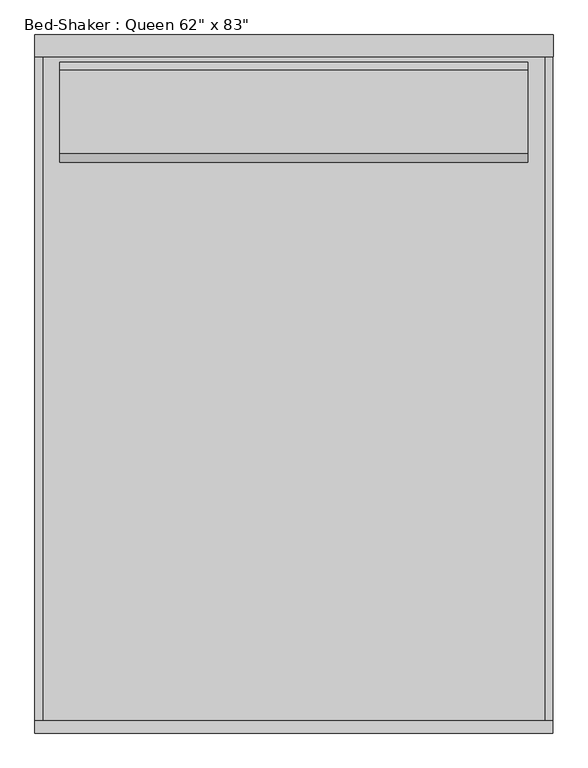
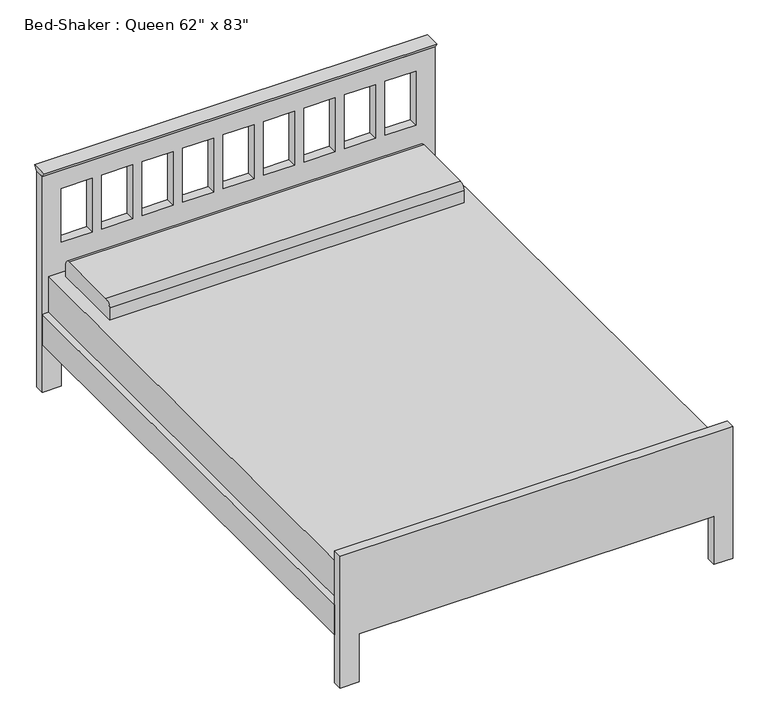
"""IFC4 building model written with IfcOpenShell, lengths in millimetres: furniture geometry."""

from ifc_helpers import new_model, si_unit, point, frame, frame_2d, origin, place, context, project, spatial, polyline, circle_curve, trimmed, segment, composite_curve, outline, extrude, source, transform, mapped, element, save


def furniture_35c09872(model_context):
    return source(origin(), model_context, "Body", "SweptSolid", [
        extrude(outline(polyline([(-38.1, 914.4), (-51.9545455, 933.45), (13.8545455, 933.45), (0.0, 914.4), (-38.1, 914.4)])), frame((-806.2365546, 0.0, 0.0), z_axis=(1.0, 0.0, 0.0), x_axis=(0.0, 1.0, 0.0)), (0.0, 0.0, 1.0), 1574.8533613),
        extrude(outline(composite_curve([segment(polyline([(-373.2486637, 482.6), (-373.2486637, 533.4)]), True, "CONTINUOUS"), segment(trimmed(circle_curve(frame_2d((-347.8486637, 533.4)), 25.4), [point((-373.2486637, 533.4))], [point((-347.8486637, 558.8))], False, "CARTESIAN"), True, "CONTINUOUS"), segment(polyline([(-347.8486637, 558.8), (-93.8486637, 558.8)]), True, "CONTINUOUS"), segment(trimmed(circle_curve(frame_2d((-93.8486637, 533.4)), 25.4), [point((-93.8486637, 558.8))], [point((-68.4486637, 533.4))], False, "CARTESIAN"), True, "CONTINUOUS"), segment(polyline([(-68.4486637, 533.4), (-68.4486637, 482.6), (-373.2486637, 482.6)]), True, "CONTINUOUS")], self_intersect=False)), frame((-730.25, 0.0, 0.0), z_axis=(1.0, 0.0, 0.0), x_axis=(0.0, 1.0, 0.0)), (0.0, 0.0, 1.0), 1422.4),
        extrude(outline(polyline([(742.95, -38.1), (742.95, -2070.1), (-781.05, -2070.1), (-781.05, -38.1), (742.95, -38.1)])), frame((0.0, 0.0, 228.6), z_axis=(0.0, 0.0, 1.0), x_axis=(1.0, 0.0, 0.0)), (0.0, 0.0, 1.0), 254.0),
        extrude(outline(polyline([(742.95, -2070.1), (742.95, -38.1), (768.35, -38.1), (768.35, -2070.1), (742.95, -2070.1)])), frame((0.0, 0.0, 203.0994861), z_axis=(0.0, 0.0, 1.0), x_axis=(1.0, 0.0, 0.0)), (0.0, 0.0, 1.0), 127.0),
        extrude(outline(polyline([(-806.45, -2070.1), (-806.45, -38.1), (-781.05, -38.1), (-781.05, -2070.1), (-806.45, -2070.1)])), frame((0.0, 0.0, 203.5755296), z_axis=(0.0, 0.0, 1.0), x_axis=(1.0, 0.0, 0.0)), (0.0, 0.0, 1.0), 127.0),
        extrude(outline(polyline([(0.0, -730.25), (203.2, -730.25), (203.2, 692.15), (0.0, 692.15), (0.0, 768.35), (558.8, 768.35), (558.8, -806.45), (0.0, -806.45), (0.0, -730.25)])), frame((0.0, -2108.2, 0.0), z_axis=(0.0, 1.0, 0.0), x_axis=(0.0, 0.0, 1.0)), (0.0, 0.0, 1.0), 38.1),
        extrude(outline(polyline([(914.4, 768.6168067), (914.4, -806.2365546), (0.0, -806.2365546), (0.0, -730.25), (203.2, -730.25), (203.2, 692.15), (0.0, 692.15), (0.0, 768.6168067), (914.4, 768.6168067)]), holes=[polyline([(838.2, -606.0722222), (609.6, -606.0722222), (609.6, -730.25), (838.2, -730.25), (838.2, -606.0722222)]), polyline([(838.2, -443.7944444), (609.6, -443.7944444), (609.6, -567.9722222), (838.2, -567.9722222), (838.2, -443.7944444)]), polyline([(838.2, -281.5166667), (609.6, -281.5166667), (609.6, -405.6944444), (838.2, -405.6944444), (838.2, -281.5166667)]), polyline([(838.2, -119.2388889), (609.6, -119.2388889), (609.6, -243.4166667), (838.2, -243.4166667), (838.2, -119.2388889)]), polyline([(838.2, 205.3166667), (609.6, 205.3166667), (609.6, 81.1388889), (838.2, 81.1388889), (838.2, 205.3166667)]), polyline([(838.2, 367.5944444), (609.6, 367.5944444), (609.6, 243.4166667), (838.2, 243.4166667), (838.2, 367.5944444)]), polyline([(838.2, 529.8722222), (609.6, 529.8722222), (609.6, 405.6944444), (838.2, 405.6944444), (838.2, 529.8722222)]), polyline([(838.2, 692.15), (609.6, 692.15), (609.6, 567.9722222), (838.2, 567.9722222), (838.2, 692.15)]), polyline([(838.2, 43.0388889), (609.6, 43.0388889), (609.6, -81.1388889), (838.2, -81.1388889), (838.2, 43.0388889)])]), frame((0.0, -38.1, 0.0), z_axis=(0.0, 1.0, 0.0), x_axis=(0.0, 0.0, 1.0)), (0.0, 0.0, 1.0), 38.1),
    ])


if __name__ == "__main__":
    model = new_model("IFC4")
    model_context = context("Model", 3, world=origin())
    ifc_project = project(units=[si_unit("LENGTHUNIT", "METRE", prefix="MILLI")], contexts=[model_context])
    site = spatial("IfcSite", under=ifc_project)
    building = spatial("IfcBuilding", under=site)
    placement = place(None, origin())
    furniture_shape = furniture_35c09872(model_context)
    element("IfcFurniture", 1, ObjectType="Bed-Shaker : Queen 62\" x 83\"", at=placement, inside=building, context=model_context, shape_type="MappedRepresentation", body=[
        mapped(furniture_shape, transform((0.0, 0.0, 0.0), x_axis=(1.0, 0.0, 0.0), y_axis=(0.0, 1.0, 0.0), z_axis=(0.0, 0.0, 1.0))),
    ])
    save(model, "model.ifc")

# Revit data of these elements
# Type "Bed-Shaker : Queen 62\" x 83\""
#   Assembly Code = "E2020200"
#   Length = 6' - 11"
#   Width = 5' - 2"
#   Frame Material = Birch
#   Mattress Material = Plywood, Sheathing
#   Default Elevation = 0
# Element 1 (IfcFurniture, "Bed-Shaker : Queen 62\" x 83\"")
#   Materials on its faces: "Birch", "Plywood, Sheathing"
# Materials
#   "Birch": class "Wood", colour RGB 224 178 126, transparency 0, Description = "Betula Alleghaniensis", Cost = 0
#   "Plywood, Sheathing": class "Wood", colour RGB 212 179 113, transparency 0, Description = "Plywood, sheathing grade", Cost = 0
